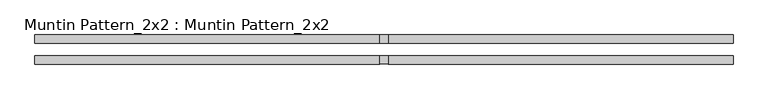
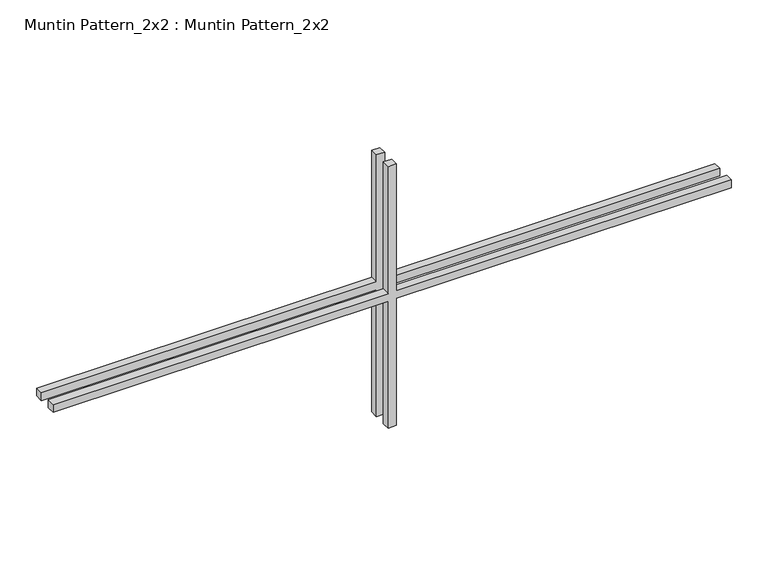
"""IFC4 building model written with IfcOpenShell, lengths in millimetres: proxy geometry, Muntin Pattern_2x2 : Muntin Pattern_2x2."""

from ifc_helpers import new_model, si_unit, frame, origin, place, context, project, spatial, polyline, outline, extrude, source, transform, mapped, element, save


def muntin_pattern_2x2_muntin_pattern_2x2_8b3f23e7(model_context):
    return source(origin(), model_context, "Body", "SweptSolid", [
        extrude(outline(polyline([(223.8375, -6.35), (223.8375, -533.4), (211.1375, -533.4), (211.1375, -6.35), (0.0, -6.35), (0.0, 6.35), (211.1375, 6.35), (211.1375, 533.4), (223.8375, 533.4), (223.8375, 6.35), (434.975, 6.35), (434.975, -6.35), (223.8375, -6.35)])), frame((0.0, 9.525, 0.0), z_axis=(0.0, 1.0, 0.0), x_axis=(0.0, 0.0, 1.0)), (0.0, 0.0, 1.0), 12.7),
        extrude(outline(polyline([(223.8375, -6.35), (223.8375, -533.4), (211.1375, -533.4), (211.1375, -6.35), (0.0, -6.35), (0.0, 6.35), (211.1375, 6.35), (211.1375, 533.4), (223.8375, 533.4), (223.8375, 6.35), (434.975, 6.35), (434.975, -6.35), (223.8375, -6.35)])), frame((0.0, -22.225, 0.0), z_axis=(0.0, 1.0, 0.0), x_axis=(0.0, 0.0, 1.0)), (0.0, 0.0, 1.0), 12.7),
    ])


if __name__ == "__main__":
    model = new_model("IFC4")
    model_context = context("Model", 3, world=origin())
    ifc_project = project(units=[si_unit("LENGTHUNIT", "METRE", prefix="MILLI")], contexts=[model_context])
    site = spatial("IfcSite", under=ifc_project)
    building = spatial("IfcBuilding", under=site)
    placement = place(None, origin())
    muntin_pattern_2x2_muntin_pattern_2x2_shape = muntin_pattern_2x2_muntin_pattern_2x2_8b3f23e7(model_context)
    element("IfcBuildingElementProxy", 1, Name="Muntin Pattern_2x2 : Muntin Pattern_2x2", ObjectType="Muntin Pattern_2x2 : Muntin Pattern_2x2", at=placement, inside=building, context=model_context, shape_type="MappedRepresentation", body=[
        mapped(muntin_pattern_2x2_muntin_pattern_2x2_shape, transform((0.0, 0.0, 0.0), x_axis=(1.0, 0.0, 0.0), y_axis=(0.0, 1.0, 0.0), z_axis=(0.0, 0.0, 1.0))),
    ])
    save(model, "model.ifc")

# Revit data of these elements
# Type "Muntin Pattern_2x2 : Muntin Pattern_2x2"
#   Width [instance default] = 4' - 0"
#   Thickness = 0' - 0 1/2"
#   Height [instance default] = 4' - 0"
#   Distance = 0' - 0 3/4"
#   Interior Material [instance default] = none
#   Exterior Material [instance default] = none
#   Default Elevation = 0
# Element 1 (IfcBuildingElementProxy, "Muntin Pattern_2x2 : Muntin Pattern_2x2")
#   Width = 3' - 6"
#   Height = 1' - 5 1/8"
#   Interior Material = Wood - Stained
#   Exterior Material = Clad - White
#   Materials on its faces: "Clad - White", "Wood - Stained"
# Materials
#   "Clad - White": class "Wood", colour RGB 242 242 238, transparency 0, Cost = 0
#   "Wood - Stained": class "Wood", colour RGB 224 178 126, transparency 0, Cost = 0
